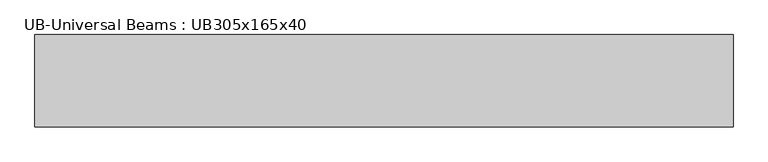
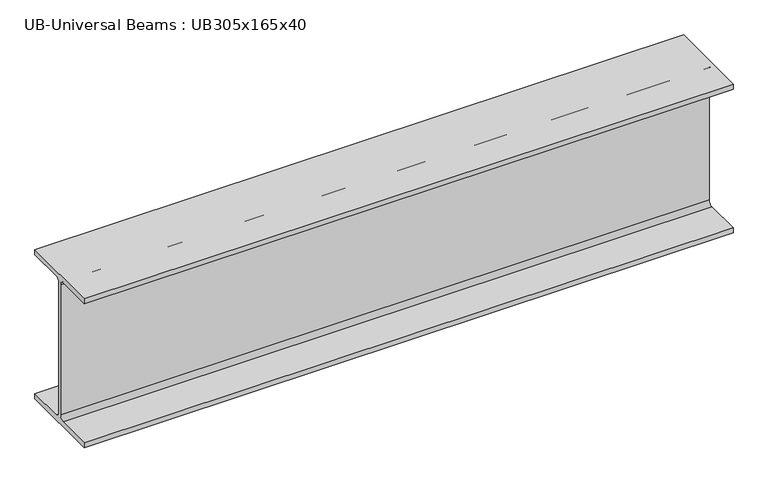
"""IFC4 building model written with IfcOpenShell, lengths in millimetres: beam geometry, UB-Universal Beams : UB305x165x40."""

from ifc_helpers import new_model, si_unit, point, frame, frame_2d, origin, place, context, project, spatial, polyline, circle_curve, trimmed, segment, composite_curve, outline, extrude, source, transform, mapped, element, save


def ub_universal_beams_ub305x165x40_2f8ff02f(model_context):
    return source(origin(), model_context, "Body", "SweptSolid", [
        extrude(outline(composite_curve([segment(polyline([(82.5, -141.5), (82.5, -151.7), (-82.5, -151.7), (-82.5, -141.5), (-11.9, -141.5)]), True, "CONTINUOUS"), segment(trimmed(circle_curve(frame_2d((-11.9, -132.6)), 8.9), [point((-11.9, -141.5))], [point((-3.0, -132.6))], True, "CARTESIAN"), True, "CONTINUOUS"), segment(polyline([(-3.0, -132.6), (-3.0, 132.6)]), True, "CONTINUOUS"), segment(trimmed(circle_curve(frame_2d((-11.9, 132.6)), 8.9), [point((-3.0, 132.6))], [point((-11.9, 141.5))], True, "CARTESIAN"), True, "CONTINUOUS"), segment(polyline([(-11.9, 141.5), (-82.5, 141.5), (-82.5, 151.7), (82.5, 151.7), (82.5, 141.5), (11.9, 141.5)]), True, "CONTINUOUS"), segment(trimmed(circle_curve(frame_2d((11.9, 132.6)), 8.9), [point((11.9, 141.5))], [point((3.0, 132.6))], True, "CARTESIAN"), True, "CONTINUOUS"), segment(polyline([(3.0, 132.6), (3.0, -132.6)]), True, "CONTINUOUS"), segment(trimmed(circle_curve(frame_2d((11.9, -132.6)), 8.9), [point((3.0, -132.6))], [point((11.9, -141.5))], True, "CARTESIAN"), True, "CONTINUOUS"), segment(polyline([(11.9, -141.5), (82.5, -141.5)]), True, "CONTINUOUS")], self_intersect=False)), frame((-635.6, 0.0, 0.0), z_axis=(1.0, 0.0, 0.0), x_axis=(0.0, 1.0, 0.0)), (0.0, 0.0, 1.0), 1249.9),
    ])


if __name__ == "__main__":
    model = new_model("IFC4")
    model_context = context("Model", 3, world=origin())
    ifc_project = project(units=[si_unit("LENGTHUNIT", "METRE", prefix="MILLI")], contexts=[model_context])
    site = spatial("IfcSite", under=ifc_project)
    building = spatial("IfcBuilding", under=site)
    placement = place(None, origin())
    ub_universal_beams_ub305x165x40_shape = ub_universal_beams_ub305x165x40_2f8ff02f(model_context)
    element("IfcBeam", 1, ObjectType="UB-Universal Beams : UB305x165x40", at=placement, inside=building, context=model_context, shape_type="MappedRepresentation", body=[
        mapped(ub_universal_beams_ub305x165x40_shape, transform((0.0, 0.0, 0.0), x_axis=(1.0, 0.0, 0.0), y_axis=(0.0, 1.0, 0.0), z_axis=(0.0, 0.0, 1.0))),
    ])
    save(model, "model.ifc")

# Revit data of these elements
# Type "UB-Universal Beams : UB305x165x40"
#   Section Name Key = "UB305X165X40"
#   Width = 16.5 cm
#   Web Thickness = 0.6 cm
#   Web Fillet = 0.89 cm
#   Warping Constant = 164000.0 cm⁶
#   Torsional Moment of Inertia = 14.70 cm⁴
#   Section Area = 51.3 cm²
#   Plastic Modulus weak axis = 142.0 cm³
#   Plastic Modulus strong axis = 623.0 cm³
#   Nominal Weight = 40.2999 kgf/m
#   Moment of Inertia weak axis = 764.00 cm⁴
#   Moment of Inertia strong axis = 8503.00 cm⁴
#   Height = 30.34 cm
#   Flange Thickness = 1.02 cm
#   Elastic Modulus weak axis = 92.6 cm³
#   Elastic Modulus strong axis = 560.0 cm³
#   Centroid Vertical = 15.17 cm
#   Centroid Horizontal = 8.25 cm
#   Bolt Spacing = 9.0 cm
#   Length [instance default] = 1500 mm
#   Structural Material [instance default] = Metal - Steel 43-275
#   Type Comments = ""
#   Assembly Code = ""
# Element 1 (IfcBeam, "UB-Universal Beams : UB305x165x40")
#   Materials on its faces: "Metal - Steel 43-275"
# Materials
#   "Metal - Steel 43-275": class "Metal", colour RGB 247 247 247, transparency 0, Cost = 0
